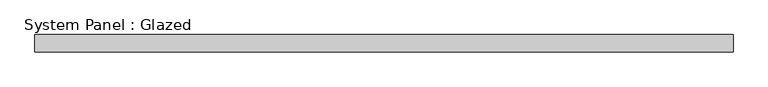
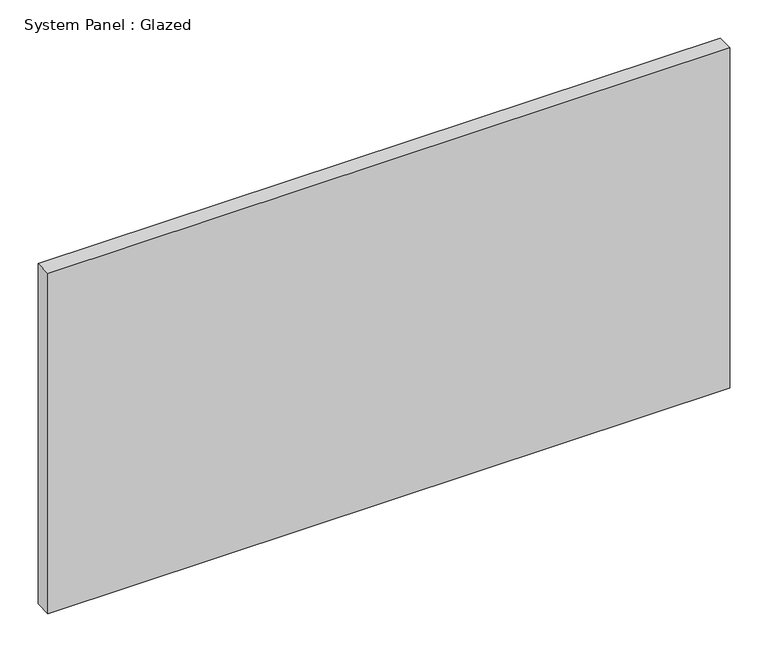
"""IFC4 building model written with IfcOpenShell, lengths in millimetres: plate geometry, System Panel : Glazed."""

from ifc_helpers import new_model, si_unit, origin, origin_with_axes, place, context, project, spatial, polyline, outline, extrude, source, transform, mapped, element, save


def system_panel_glazed_c7bdd9bd(model_context):
    return source(origin(), model_context, "Body", "SweptSolid", [
        extrude(outline(polyline([(517.525, 19.05), (-517.525, 19.05), (-517.525, 44.45), (517.525, 44.45), (517.525, 19.05)])), origin_with_axes(), (0.0, 0.0, 1.0), 546.1),
    ])


if __name__ == "__main__":
    model = new_model("IFC4")
    model_context = context("Model", 3, world=origin())
    ifc_project = project(units=[si_unit("LENGTHUNIT", "METRE", prefix="MILLI")], contexts=[model_context])
    site = spatial("IfcSite", under=ifc_project)
    building = spatial("IfcBuilding", under=site)
    placement = place(None, origin())
    system_panel_glazed_shape = system_panel_glazed_c7bdd9bd(model_context)
    element("IfcPlate", 1, ObjectType="System Panel : Glazed", at=placement, inside=building, context=model_context, shape_type="MappedRepresentation", body=[
        mapped(system_panel_glazed_shape, transform((0.0, 0.0, 0.0), x_axis=(1.0, 0.0, 0.0), y_axis=(0.0, 1.0, 0.0), z_axis=(0.0, 0.0, 1.0))),
    ])
    save(model, "model.ifc")

# Revit data of these elements
# Type "System Panel : Glazed"
#   Construction Type Id = "GSP4R"
#   Analytic Construction = "1/8 in Pilkington single glazing"
#   Visual Light Transmittance = 0.9
#   Solar Heat Gain Coefficient = 0.86
#   Heat Transfer Coefficient (U) = 1.18115 BTU/(h·ft²·°F)
#   Define Thermal Properties by = 1
# Element 1 (IfcPlate, "System Panel : Glazed")
#   Materials on its faces: "Glass"
# Materials
#   "Glass": class "Glass", colour RGB 0 128 192, transparency 0.75, Description = "Soda Lime Glass", Cost = 0
